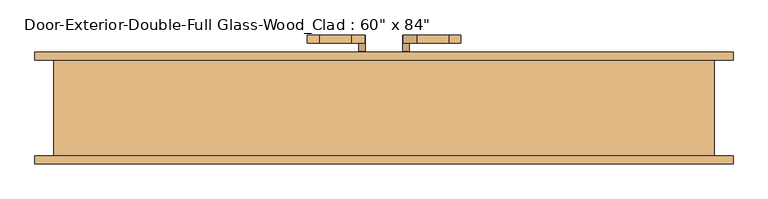
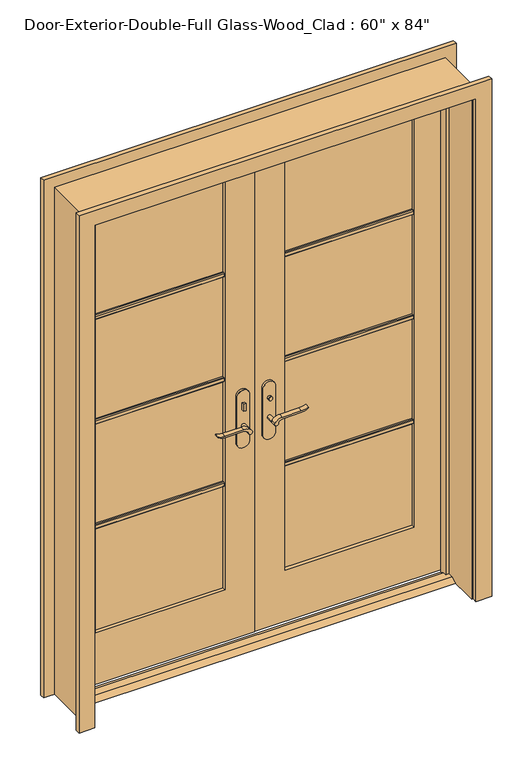
"""IFC4 building model written with IfcOpenShell, lengths in millimetres: door geometry."""

from ifc_helpers import new_model, si_unit, point, frame, frame_2d, origin, place, context, project, spatial, polyline, circle_curve, trimmed, segment, composite_curve, outline, extrude, faceted_brep, source, transform, mapped, element, save


def door_7ffae4ec(model_context):
    return source(origin(), model_context, "Body", "SolidModel", [
        extrude(outline(polyline([(19.05, 12.7), (53.975, 12.7), (79.375, 0.0), (-6.35, 0.0), (19.05, 12.7)])), frame((-762.0, 0.0, 0.0), z_axis=(1.0, 0.0, 0.0), x_axis=(0.0, 1.0, 0.0)), (0.0, 0.0, 1.0), 1524.0),
        extrude(outline(polyline([(-47.4019111, 56.2), (-57.4019111, 56.2), (-57.4019111, 66.2), (-47.4019111, 66.2), (-47.4019111, 56.2)])), frame((0.0, 0.0, 981.9), z_axis=(0.0, 0.0, 1.0), x_axis=(1.0, 0.0, 0.0)), (0.0, 0.0, 1.0), 30.0),
        extrude(outline(composite_curve([segment(trimmed(circle_curve(frame_2d((996.9, -52.4019111)), 8.0), [point((996.9, -60.4019111))], [point((996.9, -44.4019111))], False, "CARTESIAN"), True, "CONTINUOUS"), segment(trimmed(circle_curve(frame_2d((996.9, -52.4019111)), 8.0), [point((996.9, -44.4019111))], [point((996.9, -60.4019111))], False, "CARTESIAN"), True, "CONTINUOUS")], self_intersect=False)), frame((0.0, 121.125, 0.0), z_axis=(0.0, 1.0, 0.0), x_axis=(0.0, 0.0, 1.0)), (0.0, 0.0, 1.0), 10.0),
        extrude(outline(composite_curve([segment(trimmed(circle_curve(frame_2d((897.1555521, -76.0694241)), 37.2832219), [point((919.0523287, -45.8937749))], [point((934.4, -77.7693445))], False, "CARTESIAN"), True, "CONTINUOUS"), segment(polyline([(934.4, -77.7693445), (934.4, -154.045502)]), True, "CONTINUOUS"), segment(trimmed(circle_curve(frame_2d((1017.6850638, -153.9791202)), 83.2850902), [point((934.4, -154.045502))], [point((939.4, -182.4019111))], True, "CARTESIAN"), True, "CONTINUOUS"), segment(polyline([(939.4, -182.4019111), (936.6135558, -182.4019111)]), True, "CONTINUOUS"), segment(trimmed(circle_curve(frame_2d((986.6709207, -150.4622499)), 59.3791355), [point((936.6135558, -182.4019111))], [point((927.4, -154.045502))], False, "CARTESIAN"), True, "CONTINUOUS"), segment(polyline([(927.4, -154.045502), (927.4, -77.7881013)]), True, "CONTINUOUS"), segment(trimmed(circle_curve(frame_2d((909.2738613, -77.7881013)), 18.1261387), [point((927.4, -77.7881013))], [point((914.4, -60.4019111))], True, "CARTESIAN"), True, "CONTINUOUS"), segment(trimmed(circle_curve(frame_2d((914.4, -52.4019111)), 8.0), [point((914.4, -60.4019111))], [point((919.0523287, -45.8937749))], False, "CARTESIAN"), True, "CONTINUOUS")], self_intersect=False)), frame((0.0, 16.2, 0.0), z_axis=(0.0, 1.0, 0.0), x_axis=(0.0, 0.0, 1.0)), (0.0, 0.0, 1.0), 20.0),
        extrude(outline(composite_curve([segment(trimmed(circle_curve(frame_2d((914.4, -52.4019111)), 8.0), [point((914.3999903, -60.4019111))], [point((919.0523287, -45.8937749))], False, "CARTESIAN"), True, "CONTINUOUS"), segment(trimmed(circle_curve(frame_2d((897.1555521, -76.0694241)), 37.2832219), [point((919.0523287, -45.8937749))], [point((934.4, -77.7693445))], False, "CARTESIAN"), True, "CONTINUOUS"), segment(polyline([(934.4, -77.7693445), (934.4, -154.045502)]), True, "CONTINUOUS"), segment(trimmed(circle_curve(frame_2d((1017.6850638, -153.9791202)), 83.2850902), [point((934.4, -154.045502))], [point((939.4, -182.4019111))], True, "CARTESIAN"), True, "CONTINUOUS"), segment(polyline([(939.4, -182.4019111), (936.6135558, -182.4019111)]), True, "CONTINUOUS"), segment(trimmed(circle_curve(frame_2d((986.6709207, -150.4622499)), 59.3791355), [point((936.6135558, -182.4019111))], [point((927.4, -154.045502))], False, "CARTESIAN"), True, "CONTINUOUS"), segment(polyline([(927.4, -154.045502), (927.4, -77.788099)]), True, "CONTINUOUS"), segment(trimmed(circle_curve(frame_2d((909.2738682, -77.788099)), 18.1261318), [point((927.4, -77.788099))], [point((914.3999903, -60.4019111))], True, "CARTESIAN"), True, "CONTINUOUS")], self_intersect=False)), frame((0.0, 151.125, 0.0), z_axis=(0.0, 1.0, 0.0), x_axis=(0.0, 0.0, 1.0)), (0.0, 0.0, 1.0), 20.0),
        extrude(outline(composite_curve([segment(trimmed(circle_curve(frame_2d((914.4, -52.4019111)), 8.0), [point((914.4, -60.4019111))], [point((914.4, -44.4019111))], False, "CARTESIAN"), True, "CONTINUOUS"), segment(trimmed(circle_curve(frame_2d((914.4, -52.4019111)), 8.0), [point((914.4, -44.4019111))], [point((914.4, -60.4019111))], False, "CARTESIAN"), True, "CONTINUOUS")], self_intersect=False)), frame((0.0, 36.2, 0.0), z_axis=(0.0, 1.0, 0.0), x_axis=(0.0, 0.0, 1.0)), (0.0, 0.0, 1.0), 30.0),
        extrude(outline(composite_curve([segment(trimmed(circle_curve(frame_2d((914.4, -52.4019111)), 8.0), [point((914.4, -60.4019111))], [point((914.4, -44.4019111))], False, "CARTESIAN"), True, "CONTINUOUS"), segment(trimmed(circle_curve(frame_2d((914.4, -52.4019111)), 8.0), [point((914.4, -44.4019111))], [point((914.4, -60.4019111))], False, "CARTESIAN"), True, "CONTINUOUS")], self_intersect=False)), frame((0.0, 121.125, 0.0), z_axis=(0.0, 1.0, 0.0), x_axis=(0.0, 0.0, 1.0)), (0.0, 0.0, 1.0), 30.0),
        extrude(outline(composite_curve([segment(polyline([(844.4, -27.4019111), (1039.4, -27.4019111)]), True, "CONTINUOUS"), segment(trimmed(circle_curve(frame_2d((1039.4, -52.4019111)), 25.0), [point((1039.4, -27.4019111))], [point((1039.4, -77.4019111))], False, "CARTESIAN"), True, "CONTINUOUS"), segment(polyline([(1039.4, -77.4019111), (844.4, -77.4019111)]), True, "CONTINUOUS"), segment(trimmed(circle_curve(frame_2d((844.4, -52.4019111)), 25.0), [point((844.4, -77.4019111))], [point((844.4, -27.4019111))], False, "CARTESIAN"), True, "CONTINUOUS")], self_intersect=False)), frame((0.0, 66.2, 0.0), z_axis=(0.0, 1.0, 0.0), x_axis=(0.0, 0.0, 1.0)), (0.0, 0.0, 1.0), 10.0),
        extrude(outline(composite_curve([segment(polyline([(844.4, -27.4019111), (1039.4, -27.4019111)]), True, "CONTINUOUS"), segment(trimmed(circle_curve(frame_2d((1039.4, -52.4019111)), 25.0), [point((1039.4, -27.4019111))], [point((1039.4, -77.4019111))], False, "CARTESIAN"), True, "CONTINUOUS"), segment(polyline([(1039.4, -77.4019111), (844.4, -77.4019111)]), True, "CONTINUOUS"), segment(trimmed(circle_curve(frame_2d((844.4, -52.4019111)), 25.0), [point((844.4, -77.4019111))], [point((844.4, -27.4019111))], False, "CARTESIAN"), True, "CONTINUOUS")], self_intersect=False)), frame((0.0, 111.125, 0.0), z_axis=(0.0, 1.0, 0.0), x_axis=(0.0, 0.0, 1.0)), (0.0, 0.0, 1.0), 10.0),
        extrude(outline(polyline([(47.3875, 131.125), (57.3875, 131.125), (57.3875, 121.125), (47.3875, 121.125), (47.3875, 131.125)])), frame((0.0, 0.0, 981.9), z_axis=(0.0, 0.0, 1.0), x_axis=(1.0, 0.0, 0.0)), (0.0, 0.0, 1.0), 30.0),
        extrude(outline(composite_curve([segment(trimmed(circle_curve(frame_2d((996.9, 52.3875)), 8.0), [point((996.9, 60.3875))], [point((996.9, 44.3875))], False, "CARTESIAN"), True, "CONTINUOUS"), segment(trimmed(circle_curve(frame_2d((996.9, 52.3875)), 8.0), [point((996.9, 44.3875))], [point((996.9, 60.3875))], False, "CARTESIAN"), True, "CONTINUOUS")], self_intersect=False)), frame((0.0, 56.2, 0.0), z_axis=(0.0, 1.0, 0.0), x_axis=(0.0, 0.0, 1.0)), (0.0, 0.0, 1.0), 10.0),
        extrude(outline(composite_curve([segment(trimmed(circle_curve(frame_2d((914.4, 52.3875)), 8.0), [point((919.0523287, 45.8793637))], [point((914.4, 60.3875))], False, "CARTESIAN"), True, "CONTINUOUS"), segment(trimmed(circle_curve(frame_2d((909.2738613, 77.7736901)), 18.1261387), [point((914.4, 60.3875))], [point((927.4, 77.7736901))], True, "CARTESIAN"), True, "CONTINUOUS"), segment(polyline([(927.4, 77.7736901), (927.4, 154.0310909)]), True, "CONTINUOUS"), segment(trimmed(circle_curve(frame_2d((986.6709207, 150.4478388)), 59.3791355), [point((927.4, 154.0310909))], [point((936.6135558, 182.3875))], False, "CARTESIAN"), True, "CONTINUOUS"), segment(polyline([(936.6135558, 182.3875), (939.4, 182.3875)]), True, "CONTINUOUS"), segment(trimmed(circle_curve(frame_2d((1017.6850638, 153.9647091)), 83.2850902), [point((939.4, 182.3875))], [point((934.4, 154.0310909))], True, "CARTESIAN"), True, "CONTINUOUS"), segment(polyline([(934.4, 154.0310909), (934.4, 77.7549333)]), True, "CONTINUOUS"), segment(trimmed(circle_curve(frame_2d((897.1555521, 76.0550129)), 37.2832219), [point((934.4, 77.7549333))], [point((919.0523287, 45.8793637))], False, "CARTESIAN"), True, "CONTINUOUS")], self_intersect=False)), frame((0.0, 151.125, 0.0), z_axis=(0.0, 1.0, 0.0), x_axis=(0.0, 0.0, 1.0)), (0.0, 0.0, 1.0), 20.0),
        extrude(outline(composite_curve([segment(trimmed(circle_curve(frame_2d((909.2738682, 77.7736878)), 18.1261318), [point((914.3999903, 60.3875))], [point((927.4, 77.7736878))], True, "CARTESIAN"), True, "CONTINUOUS"), segment(polyline([(927.4, 77.7736878), (927.4, 154.0310909)]), True, "CONTINUOUS"), segment(trimmed(circle_curve(frame_2d((986.6709207, 150.4478388)), 59.3791355), [point((927.4, 154.0310909))], [point((936.6135558, 182.3875))], False, "CARTESIAN"), True, "CONTINUOUS"), segment(polyline([(936.6135558, 182.3875), (939.4, 182.3875)]), True, "CONTINUOUS"), segment(trimmed(circle_curve(frame_2d((1017.6850638, 153.9647091)), 83.2850902), [point((939.4, 182.3875))], [point((934.4, 154.0310909))], True, "CARTESIAN"), True, "CONTINUOUS"), segment(polyline([(934.4, 154.0310909), (934.4, 77.7549333)]), True, "CONTINUOUS"), segment(trimmed(circle_curve(frame_2d((897.1555521, 76.0550129)), 37.2832219), [point((934.4, 77.7549333))], [point((919.0523287, 45.8793637))], False, "CARTESIAN"), True, "CONTINUOUS"), segment(trimmed(circle_curve(frame_2d((914.4, 52.3875)), 8.0), [point((919.0523287, 45.8793637))], [point((914.3999903, 60.3875))], False, "CARTESIAN"), True, "CONTINUOUS")], self_intersect=False)), frame((0.0, 16.2, 0.0), z_axis=(0.0, 1.0, 0.0), x_axis=(0.0, 0.0, 1.0)), (0.0, 0.0, 1.0), 20.0),
        extrude(outline(composite_curve([segment(trimmed(circle_curve(frame_2d((914.4, 52.3875)), 8.0), [point((914.4, 60.3875))], [point((914.4, 44.3875))], False, "CARTESIAN"), True, "CONTINUOUS"), segment(trimmed(circle_curve(frame_2d((914.4, 52.3875)), 8.0), [point((914.4, 44.3875))], [point((914.4, 60.3875))], False, "CARTESIAN"), True, "CONTINUOUS")], self_intersect=False)), frame((0.0, 121.125, 0.0), z_axis=(0.0, 1.0, 0.0), x_axis=(0.0, 0.0, 1.0)), (0.0, 0.0, 1.0), 30.0),
        extrude(outline(composite_curve([segment(trimmed(circle_curve(frame_2d((914.4, 52.3875)), 8.0), [point((914.4, 60.3875))], [point((914.4, 44.3875))], False, "CARTESIAN"), True, "CONTINUOUS"), segment(trimmed(circle_curve(frame_2d((914.4, 52.3875)), 8.0), [point((914.4, 44.3875))], [point((914.4, 60.3875))], False, "CARTESIAN"), True, "CONTINUOUS")], self_intersect=False)), frame((0.0, 36.2, 0.0), z_axis=(0.0, 1.0, 0.0), x_axis=(0.0, 0.0, 1.0)), (0.0, 0.0, 1.0), 30.0),
        extrude(outline(composite_curve([segment(trimmed(circle_curve(frame_2d((844.4, 52.3875)), 25.0), [point((844.4, 27.3875))], [point((844.4, 77.3875))], False, "CARTESIAN"), True, "CONTINUOUS"), segment(polyline([(844.4, 77.3875), (1039.4, 77.3875)]), True, "CONTINUOUS"), segment(trimmed(circle_curve(frame_2d((1039.4, 52.3875)), 25.0), [point((1039.4, 77.3875))], [point((1039.4, 27.3875))], False, "CARTESIAN"), True, "CONTINUOUS"), segment(polyline([(1039.4, 27.3875), (844.4, 27.3875)]), True, "CONTINUOUS")], self_intersect=False)), frame((0.0, 111.125, 0.0), z_axis=(0.0, 1.0, 0.0), x_axis=(0.0, 0.0, 1.0)), (0.0, 0.0, 1.0), 10.0),
        extrude(outline(composite_curve([segment(trimmed(circle_curve(frame_2d((844.4, 52.3875)), 25.0), [point((844.4, 27.3875))], [point((844.4, 77.3875))], False, "CARTESIAN"), True, "CONTINUOUS"), segment(polyline([(844.4, 77.3875), (1039.4, 77.3875)]), True, "CONTINUOUS"), segment(trimmed(circle_curve(frame_2d((1039.4, 52.3875)), 25.0), [point((1039.4, 77.3875))], [point((1039.4, 27.3875))], False, "CARTESIAN"), True, "CONTINUOUS"), segment(polyline([(1039.4, 27.3875), (844.4, 27.3875)]), True, "CONTINUOUS")], self_intersect=False)), frame((0.0, 66.2, 0.0), z_axis=(0.0, 1.0, 0.0), x_axis=(0.0, 0.0, 1.0)), (0.0, 0.0, 1.0), 10.0),
        extrude(outline(polyline([(90.17, 1578.371875), (90.17, 1559.321875), (83.82, 1559.321875), (80.645, 1562.496875), (80.645, 1575.196875), (83.82, 1578.371875), (90.17, 1578.371875)])), frame((120.65, 0.0, 0.0), z_axis=(1.0, 0.0, 0.0), x_axis=(0.0, 1.0, 0.0)), (0.0, 0.0, 1.0), 520.7),
        extrude(outline(polyline([(90.17, 1132.68125), (90.17, 1113.63125), (83.82, 1113.63125), (80.645, 1116.80625), (80.645, 1129.50625), (83.82, 1132.68125), (90.17, 1132.68125)])), frame((120.65, 0.0, 0.0), z_axis=(1.0, 0.0, 0.0), x_axis=(0.0, 1.0, 0.0)), (0.0, 0.0, 1.0), 520.7),
        extrude(outline(polyline([(90.17, 686.990625), (90.17, 667.940625), (83.82, 667.940625), (80.645, 671.115625), (80.645, 683.815625), (83.82, 686.990625), (90.17, 686.990625)])), frame((120.65, 0.0, 0.0), z_axis=(1.0, 0.0, 0.0), x_axis=(0.0, 1.0, 0.0)), (0.0, 0.0, 1.0), 520.7),
        extrude(outline(polyline([(97.155, 1578.371875), (103.505, 1578.371875), (106.68, 1575.196875), (106.68, 1562.496875), (103.505, 1559.321875), (97.155, 1559.321875), (97.155, 1578.371875)])), frame((-641.35, 0.0, 0.0), z_axis=(1.0, 0.0, 0.0), x_axis=(0.0, 1.0, 0.0)), (0.0, 0.0, 1.0), 520.7),
        extrude(outline(polyline([(97.155, 1132.68125), (103.505, 1132.68125), (106.68, 1129.50625), (106.68, 1116.80625), (103.505, 1113.63125), (97.155, 1113.63125), (97.155, 1132.68125)])), frame((-641.35, 0.0, 0.0), z_axis=(1.0, 0.0, 0.0), x_axis=(0.0, 1.0, 0.0)), (0.0, 0.0, 1.0), 520.7),
        extrude(outline(polyline([(97.155, 686.990625), (103.505, 686.990625), (106.68, 683.815625), (106.68, 671.115625), (103.505, 667.940625), (97.155, 667.940625), (97.155, 686.990625)])), frame((-641.35, 0.0, 0.0), z_axis=(1.0, 0.0, 0.0), x_axis=(0.0, 1.0, 0.0)), (0.0, 0.0, 1.0), 520.7),
        extrude(outline(polyline([(97.155, 1578.371875), (103.505, 1578.371875), (106.68, 1575.196875), (106.68, 1562.496875), (103.505, 1559.321875), (97.155, 1559.321875), (97.155, 1578.371875)])), frame((120.65, 0.0, 0.0), z_axis=(1.0, 0.0, 0.0), x_axis=(0.0, 1.0, 0.0)), (0.0, 0.0, 1.0), 520.7),
        extrude(outline(polyline([(97.155, 1132.68125), (103.505, 1132.68125), (106.68, 1129.50625), (106.68, 1116.80625), (103.505, 1113.63125), (97.155, 1113.63125), (97.155, 1132.68125)])), frame((120.65, 0.0, 0.0), z_axis=(1.0, 0.0, 0.0), x_axis=(0.0, 1.0, 0.0)), (0.0, 0.0, 1.0), 520.7),
        extrude(outline(polyline([(97.155, 686.990625), (103.505, 686.990625), (106.68, 683.815625), (106.68, 671.115625), (103.505, 667.940625), (97.155, 667.940625), (97.155, 686.990625)])), frame((120.65, 0.0, 0.0), z_axis=(1.0, 0.0, 0.0), x_axis=(0.0, 1.0, 0.0)), (0.0, 0.0, 1.0), 520.7),
        extrude(outline(polyline([(90.17, 1578.371875), (90.17, 1559.321875), (83.82, 1559.321875), (80.645, 1562.496875), (80.645, 1575.196875), (83.82, 1578.371875), (90.17, 1578.371875)])), frame((-641.35, 0.0, 0.0), z_axis=(1.0, 0.0, 0.0), x_axis=(0.0, 1.0, 0.0)), (0.0, 0.0, 1.0), 520.7),
        extrude(outline(polyline([(90.17, 1132.68125), (90.17, 1113.63125), (83.82, 1113.63125), (80.645, 1116.80625), (80.645, 1129.50625), (83.82, 1132.68125), (90.17, 1132.68125)])), frame((-641.35, 0.0, 0.0), z_axis=(1.0, 0.0, 0.0), x_axis=(0.0, 1.0, 0.0)), (0.0, 0.0, 1.0), 520.7),
        extrude(outline(polyline([(90.17, 686.990625), (90.17, 667.940625), (83.82, 667.940625), (80.645, 671.115625), (80.645, 683.815625), (83.82, 686.990625), (90.17, 686.990625)])), frame((-641.35, 0.0, 0.0), z_axis=(1.0, 0.0, 0.0), x_axis=(0.0, 1.0, 0.0)), (0.0, 0.0, 1.0), 520.7),
        extrude(outline(polyline([(0.0, 768.35), (0.0, 831.85), (2203.45, 831.85), (2203.45, -831.85), (0.0, -831.85), (0.0, -768.35), (2139.95, -768.35), (2139.95, 768.35), (0.0, 768.35)])), frame((0.0, -136.525, 0.0), z_axis=(0.0, 1.0, 0.0), x_axis=(0.0, 0.0, 1.0)), (0.0, 0.0, 1.0), 19.05),
        extrude(outline(polyline([(0.0, 768.35), (0.0, 831.85), (2203.45, 831.85), (2203.45, -831.85), (0.0, -831.85), (0.0, -768.35), (2139.95, -768.35), (2139.95, 768.35), (0.0, 768.35)])), frame((0.0, 111.125, 0.0), z_axis=(0.0, 1.0, 0.0), x_axis=(0.0, 0.0, 1.0)), (0.0, 0.0, 1.0), 19.05),
        faceted_brep([(787.4, 111.125, 0.0), (787.4, -117.475, 0.0), (762.0, -117.475, 0.0), (762.0, 41.275, 0.0), (749.3, 41.275, 0.0), (749.3, 76.2, 0.0), (762.0, 76.2, 0.0), (762.0, 111.125, 0.0), (787.4, 111.125, 2159.0), (787.4, -117.475, 2159.0), (-787.4, -117.475, 2159.0), (-787.4, -117.475, 0.0), (-762.0, -117.475, 0.0), (-762.0, -117.475, 2133.6), (762.0, -117.475, 2133.6), (762.0, 41.275, 2133.6), (-762.0, 41.275, 2133.6), (-762.0, 41.275, 0.0), (-749.3, 41.275, 0.0), (-749.3, 41.275, 2120.9), (749.3, 41.275, 2120.9), (749.3, 76.2, 2120.9), (1.5875, 76.2, 2120.9), (-1.6019111, 76.2, 2120.9), (-749.3, 76.2, 2120.9), (-749.3, 76.2, 0.0), (-762.0, 76.2, 0.0), (-762.0, 76.2, 2133.6), (-1.6019111, 76.2, 2133.6), (1.5875, 76.2, 2133.6), (762.0, 76.2, 2133.6), (762.0, 111.125, 2133.6), (1.5875, 111.125, 2133.6), (-1.6019111, 111.125, 2133.6), (-762.0, 111.125, 2133.6), (-762.0, 111.125, 0.0), (-787.4, 111.125, 0.0), (-787.4, 111.125, 2159.0)], [[[0, 1, 2, 3, 4, 5, 6, 7]], [[1, 0, 8, 9]], [[2, 1, 9, 10, 11, 12, 13, 14]], [[3, 2, 14, 15]], [[4, 3, 15, 16, 17, 18, 19, 20]], [[5, 4, 20, 21]], [[6, 5, 21, 22, 23, 24, 25, 26, 27, 28, 29, 30]], [[7, 6, 30, 31]], [[0, 7, 31, 32, 33, 34, 35, 36, 37, 8]], [[9, 8, 37, 10]], [[14, 13, 16, 15]], [[20, 19, 24, 23, 22, 21]], [[31, 30, 29, 28, 27, 34, 33, 32]], [[12, 11, 36, 35, 26, 25, 18, 17]], [[11, 10, 37, 36]], [[13, 12, 17, 16]], [[19, 18, 25, 24]], [[27, 26, 35, 34]]]),
        extrude(outline(polyline([(12.7, 762.0), (2133.6, 762.0), (2133.6, 1.5875), (12.7, 1.5875), (12.7, 762.0)]), holes=[polyline([(2014.5375, 120.65), (2014.5375, 641.35), (231.775, 641.35), (231.775, 120.65), (2014.5375, 120.65)])]), frame((0.0, 76.2, 0.0), z_axis=(0.0, 1.0, 0.0), x_axis=(0.0, 0.0, 1.0)), (0.0, 0.0, 1.0), 34.925),
        extrude(outline(polyline([(2133.6, -762.0), (12.7, -762.0), (12.7, -1.6019111), (2133.6, -1.6019111), (2133.6, -762.0)]), holes=[polyline([(231.775, -641.35), (2014.5375, -641.35), (2014.5375, -120.65), (231.775, -120.65), (231.775, -641.35)])]), frame((0.0, 76.2, 0.0), z_axis=(0.0, 1.0, 0.0), x_axis=(0.0, 0.0, 1.0)), (0.0, 0.0, 1.0), 34.925),
        extrude(outline(polyline([(641.35, 90.17), (120.65, 90.17), (120.65, 97.155), (641.35, 97.155), (641.35, 90.17)])), frame((0.0, 0.0, 231.775), z_axis=(0.0, 0.0, 1.0), x_axis=(1.0, 0.0, 0.0)), (0.0, 0.0, 1.0), 1782.7625),
        extrude(outline(polyline([(-120.65, 90.17), (-641.35, 90.17), (-641.35, 97.155), (-120.65, 97.155), (-120.65, 90.17)])), frame((0.0, 0.0, 231.775), z_axis=(0.0, 0.0, 1.0), x_axis=(1.0, 0.0, 0.0)), (0.0, 0.0, 1.0), 1782.7625),
    ])


if __name__ == "__main__":
    model = new_model("IFC4")
    model_context = context("Model", 3, world=origin())
    ifc_project = project(units=[si_unit("LENGTHUNIT", "METRE", prefix="MILLI")], contexts=[model_context])
    site = spatial("IfcSite", under=ifc_project)
    building = spatial("IfcBuilding", under=site)
    placement = place(None, origin())
    door_shape = door_7ffae4ec(model_context)
    element("IfcDoor", 1, ObjectType="Door-Exterior-Double-Full Glass-Wood_Clad : 60\" x 84\"", at=placement, inside=building, context=model_context, shape_type="MappedRepresentation", body=[
        mapped(door_shape, transform((0.0, 0.0, 0.0), x_axis=(1.0, 0.0, 0.0), y_axis=(0.0, 1.0, 0.0), z_axis=(0.0, 0.0, 1.0))),
    ])
    save(model, "model.ifc")

# Revit data of these elements
# Type "Door-Exterior-Double-Full Glass-Wood_Clad : 60\" x 84\""
#   Type Mark = "18"
#   Assembly Code = "B2030100"
#   Analytic Construction = "French door, wood frame with double glass"
#   Top Rail = 0' - 4 11/16"
#   Threshold Offset [instance default] = 0' - 0 1/2"
#   Thickness = 0' - 1 3/8"
#   Thermal Resistance (R) = 1.9158 (h·ft²·°F)/BTU
#   Swing Angle [instance default] = 90.00°
#   Stiles = 0' - 4 3/4"
#   Rough Width = 5' - 2"
#   Rough Height = 7' - 1"
#   Panel Width = 2' - 6"
#   Door Offset [instance default] = 0' - 0"
#   Height = 7' - 0"
#   Width = 5' - 0"
#   Heat Transfer Coefficient (U) = 0.5220 BTU/(h·ft²·°F)
#   Bottom Rail = 0' - 9 1/8"
#   Exterior Trim [instance default] = yes
#   Threshold [instance default] = yes
#   Show Grill [instance default] = yes
#   Function = 1
#   Trim Material = Cherry
#   Threshold Material = Cherry
#   Panel Material = Cherry
#   Glazing = Glass
#   Frame Material = Cherry
#   Door Handle Material = Aluminum
#   Visual Light Transmittance = 0
#   Solar Heat Gain Coefficient = 0
#   Wall Closure = (empty or 0)
#   Construction Type = (empty or 0)
# Element 1 (IfcDoor, "Door-Exterior-Double-Full Glass-Wood_Clad : 60\" x 84\"")
#   Materials on its faces: "Cherry", "Aluminum", "Glass"
# Materials
#   "Cherry": class "Wood", colour RGB 226 177 128, transparency 0, Description = "Prunus Serotina", Cost = 0
#   "Glass": class "Glass", colour RGB 0 128 192, transparency 0.75, Description = "Soda Lime Glass", Cost = 0
#   "Aluminum": class "Metal", colour RGB 247 247 247, transparency 0, Description = "Aluminum 6061", Cost = 0
